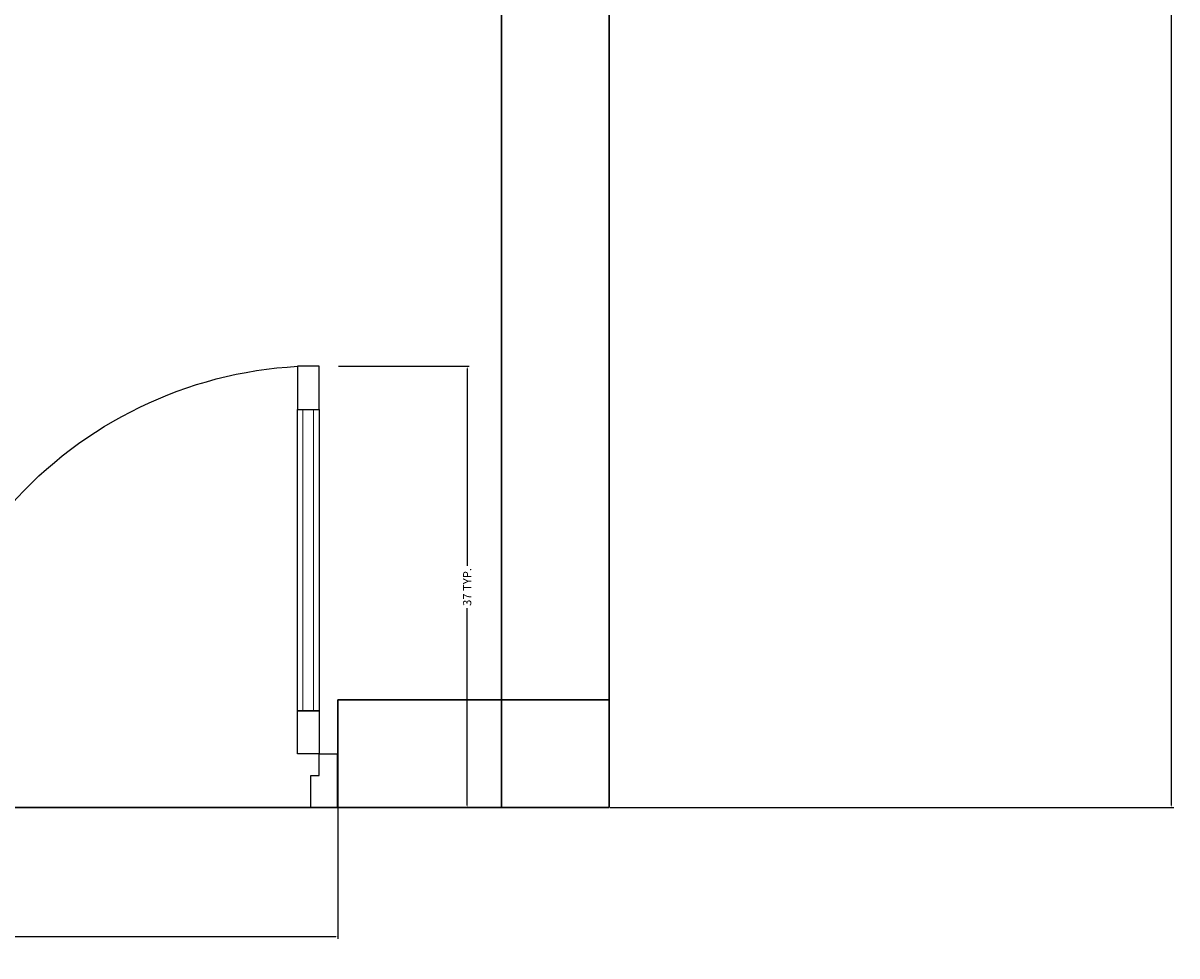
# Model space of a CAD drawing. Units: inches. Extents: x 867 to 1667, y -234 to 788.
# Tile 20 of 42: x 1571 to 1667, y -199 to -121. Entities that reach past the tile are written whole.
import ezdxf

# ---------------------------------------------------------------- set-up
doc = ezdxf.new("R2010")
doc.units = ezdxf.units.IN
doc.header["$MEASUREMENT"] = 0
for name, color, linetype, lineweight in [('A-ANNO-DIMS', 2, 'Continuous', 18), ('A-Door', 150, 'Continuous', 25), ('A-Glaz', 92, 'Continuous', 18), ('A-Wall', 7, 'Continuous', 35), ('A-WALL-SITE', 8, 'Continuous', 30)]:
    doc.layers.add(name, color=color, linetype=linetype, lineweight=lineweight)
doc.layers.add('NT', color=1, linetype='Continuous')
doc.styles.get("Standard").update_dxf_attribs({"font": 'arial.ttf'})
doc.dimstyles.get("Standard").update_dxf_attribs({"dimtxt": 0.6875, "dimasz": 0.18, "dimexe": 0.18, "dimexo": 0.0625, "dimgap": 0.09, "dimtad": 0, "dimdec": 4, "dimzin": 0, "dimdsep": 46, "dimlunit": 4, "dimtxsty": 'Standard', "dimcen": 0.09, "dimadec": 0, "dimazin": 0, "dimtfac": 1, "dimtdec": 4, "dimtofl": 0, "dimtmove": 0, "dimatfit": 3, "dimfxl": 1, "dimtolj": 1, "dimtzin": 0, "dimarcsym": 0})

# ---------------------------------------------------------------- blocks, each defined once
blk = doc.blocks.new('A$C0EE93B68')
at = {"layer": 'A-Door'}
for points in [[(100, 1565), (100, 1600), (0, 1600), (0, 1550), (50, 1550), (60, 1550), (60, 1565)], [(100, 1525), (180, 1525), (180, 1565), (100, 1565)], [(180, 1525), (740, 1525), (740, 1565), (180, 1565)], [(820, 1525), (740, 1525), (740, 1565), (820, 1565)], [(100, 75), (180, 75), (180, 35), (100, 35)], [(180, 75), (740, 75), (740, 35), (180, 35)], [(820, 75), (740, 75), (740, 35), (820, 35)], [(100, 35), (100, 0), (0, 0), (0, 50), (50, 50), (60, 50), (60, 35)]]:
    blk.add_lwpolyline(points, close=True, dxfattribs=at)
at = {"layer": 'A-Glaz'}
for points in [[(180, 1535), (740, 1535), (740, 1555), (180, 1555)], [(180, 65), (740, 65), (740, 45), (180, 45)]]:
    blk.add_lwpolyline(points, close=True, dxfattribs=at)
at = {"layer": 'A-Wall'}
for p, q in [((0, 1600), (100, 1600)), ((0, 0), (100, 0))]:
    blk.add_line(p, q, dxfattribs=at)
at = {"layer": 'NT'}
for centre, start, end in [((51.6, 1567.9), 266.1547, 356.8081), ((51.6, 32.1), 3.1919, 93.8453)]:
    blk.add_arc(centre, 769.6, start, end, dxfattribs=at)
blk = doc.blocks.new('*D9')
at = {"layer": 'A-ANNO-DIMS', "color": 0, "lineweight": -2, "transparency": 16777216}
for p, q in [((1525.265, -186.471), (1525.265, -197.382)), ((1597.224, -186.471), (1597.224, -197.382)), ((1525.445, -197.202), (1558.046, -197.202)), ((1597.044, -197.202), (1564.443, -197.202))]:
    blk.add_line(p, q, dxfattribs=at)
at = {"layer": 'A-ANNO-DIMS', "color": 0, "transparency": 16777216}
for points in [[(1525.445, -197.172), (1525.445, -197.232), (1525.265, -197.202)], [(1597.044, -197.172), (1597.044, -197.232), (1597.224, -197.202)]]:
    blk.add_solid(points, dxfattribs=at)
at = {"layer": 'Defpoints', "color": 0, "transparency": 16777216}
for p in [(1525.265, -186.408), (1597.224, -186.408), (1597.224, -197.202)]:
    blk.add_point(p, dxfattribs=at)
at = {"layer": 'A-ANNO-DIMS', "color": 0, "transparency": 16777216, "insert": (1561.244, -197.202), "char_height": 0.6875, "attachment_point": 5}
blk.add_mtext('\\A1;GATE 72 TYP.', dxfattribs=at)
blk = doc.blocks.new('*D10')
at = {"layer": 'A-ANNO-DIMS', "color": 0, "lineweight": -2, "transparency": 16777216}
for p, q in [((1597.286, -149.529), (1608.198, -149.529)), ((1608.018, -149.709), (1608.018, -166.206)), ((1608.018, -186.228), (1608.018, -169.732)), ((1597.286, -186.408), (1608.198, -186.408))]:
    blk.add_line(p, q, dxfattribs=at)
at = {"layer": 'A-ANNO-DIMS', "color": 0, "transparency": 16777216}
for points in [[(1607.988, -149.709), (1608.048, -149.709), (1608.018, -149.529)], [(1607.988, -186.228), (1608.048, -186.228), (1608.018, -186.408)]]:
    blk.add_solid(points, dxfattribs=at)
at = {"layer": 'Defpoints', "color": 0, "transparency": 16777216}
for p in [(1597.224, -149.529), (1608.018, -149.529), (1597.224, -186.408)]:
    blk.add_point(p, dxfattribs=at)
at = {"layer": 'A-ANNO-DIMS', "color": 0, "transparency": 16777216, "insert": (1608.018, -167.969), "char_height": 0.6875, "attachment_point": 5, "rotation": 90}
blk.add_mtext('\\A1;37 TYP.', dxfattribs=at)
blk = doc.blocks.new('*D18')
at = {"layer": 'A-ANNO-DIMS', "color": 0, "lineweight": -2, "transparency": 16777216}
for p, q in [((1619.949, 740.617), (1667.017, 740.617)), ((1666.837, 740.437), (1666.837, 277.954)), ((1666.837, -186.228), (1666.837, 276.255)), ((1619.949, -186.408), (1667.017, -186.408))]:
    blk.add_line(p, q, dxfattribs=at)
at = {"layer": 'A-ANNO-DIMS', "color": 0, "transparency": 16777216}
for points in [[(1666.807, 740.437), (1666.867, 740.437), (1666.837, 740.617)], [(1666.807, -186.228), (1666.867, -186.228), (1666.837, -186.408)]]:
    blk.add_solid(points, dxfattribs=at)
at = {"layer": 'Defpoints', "color": 0, "transparency": 16777216}
for p in [(1619.887, 740.617), (1666.837, 740.617), (1619.887, -186.408)]:
    blk.add_point(p, dxfattribs=at)
at = {"layer": 'A-ANNO-DIMS', "color": 0, "transparency": 16777216, "insert": (1666.837, 277.104), "char_height": 0.6875, "attachment_point": 5, "rotation": 90}
blk.add_mtext('\\A1;927', dxfattribs=at)

msp = doc.modelspace()

# ---------------------------------------------------------------- linework, layer by layer
at = {"layer": 'A-WALL-SITE'}
for p, q in [((1610.8866, 740.617), (1610.8866, -186.4081)), ((1619.8866, 740.617), (1619.8866, -186.4081)), ((1619.8866, -177.4081), (1597.2238, -177.4081)), ((1597.2238, -181.9107), (1597.2238, -177.4081)), ((1619.8866, -186.4081), (914.8866, -186.4081))]:
    msp.add_line(p, q, dxfattribs=at)

# ---------------------------------------------------------------- block references
at = {"layer": 'A-Door', "xscale": -0.0449743717352066, "yscale": 0.0449743717352066, "zscale": 0.0449743717352066, "rotation": 270}
msp.add_blockref('A$C0EE93B68', (1525.2648, -186.4081), dxfattribs=at)

# ---------------------------------------------------------------- dimensions: what is measured, and where the dimension line sits
at = {"layer": 'A-ANNO-DIMS'}
dim = msp.add_linear_dim(base=(1666.8366, 740.617), p1=(1619.8866, -186.4081), p2=(1619.8866, 740.617), angle=90, dimstyle='Standard', override={"dimdec": 0, "dimlfac": 1, "dimrnd": 0, "dimzin": 0, "dimdsep": 46, "dimlunit": 2}, dxfattribs=at)
dim.commit()
dim.dimension.update_dxf_attribs({"geometry": '*D18', "text_midpoint": (1666.8366, 277.1045)})
dim = msp.add_linear_dim(base=(1608.0176, -149.5291), p1=(1597.2238, -186.4081), p2=(1597.2238, -149.5291), angle=90, text='<> TYP.', dimstyle='Standard', override={"dimdec": 0, "dimlfac": 1, "dimrnd": 0, "dimzin": 0, "dimdsep": 46, "dimlunit": 2}, dxfattribs=at)
dim.commit()
dim.dimension.update_dxf_attribs({"geometry": '*D10', "text_midpoint": (1608.0176, -167.9686)})
dim = msp.add_linear_dim(base=(1597.2238, -197.2019), p1=(1525.2648, -186.4081), p2=(1597.2238, -186.4081), text='GATE <> TYP.', dimstyle='Standard', override={"dimdec": 0, "dimlfac": 1, "dimrnd": 0, "dimzin": 0, "dimdsep": 46, "dimlunit": 2}, dxfattribs=at)
dim.commit()
dim.dimension.update_dxf_attribs({"geometry": '*D9', "text_midpoint": (1561.2443, -197.2019)})

doc.saveas('drawing.dxf')
